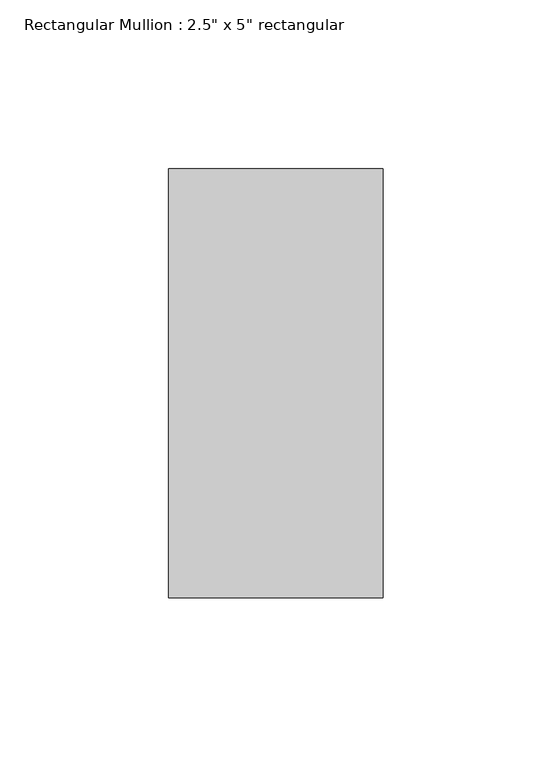
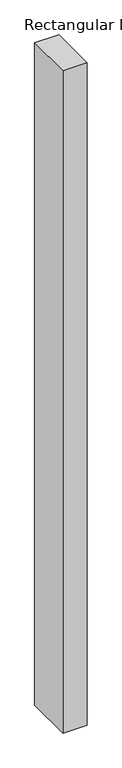
"""IFC4 building model written with IfcOpenShell, lengths in millimetres: member geometry."""

from ifc_helpers import new_model, si_unit, frame, origin, place, context, project, spatial, polyline, outline, extrude, source, transform, mapped, element, save


def member_78ce859c(model_context):
    return source(origin(), model_context, "Body", "SweptSolid", [
        extrude(outline(polyline([(31.75, 63.5), (31.75, -63.5), (-31.75, -63.5), (-31.75, 63.5), (31.75, 63.5)])), frame((0.0, 0.0, -1825.0287468), z_axis=(0.0, 0.0, 1.0), x_axis=(1.0, 0.0, 0.0)), (0.0, 0.0, 1.0), 1825.0287468),
    ])


if __name__ == "__main__":
    model = new_model("IFC4")
    model_context = context("Model", 3, world=origin())
    ifc_project = project(units=[si_unit("LENGTHUNIT", "METRE", prefix="MILLI")], contexts=[model_context])
    site = spatial("IfcSite", under=ifc_project)
    building = spatial("IfcBuilding", under=site)
    placement = place(None, origin())
    member_shape = member_78ce859c(model_context)
    element("IfcMember", 1, ObjectType="Rectangular Mullion : 2.5\" x 5\" rectangular", at=placement, inside=building, context=model_context, shape_type="MappedRepresentation", body=[
        mapped(member_shape, transform((0.0, 0.0, 0.0), x_axis=(1.0, 0.0, 0.0), y_axis=(0.0, 1.0, 0.0), z_axis=(0.0, 0.0, 1.0))),
    ])
    save(model, "model.ifc")

# Revit data of these elements
# Type "Rectangular Mullion : 2.5\" x 5\" rectangular"
#   built-in parameter 1007304 = 0.416667 (stored number, unit not read)
#   built-in parameter 1007301 = 0.104167 (stored number, unit not read)
#   built-in parameter 1007300 = 0.104167 (stored number, unit not read)
# Element 1 (IfcMember, "Rectangular Mullion : 2.5\" x 5\" rectangular")
#   Materials on its faces: "Aluminum"
# Materials
#   "Aluminum": class "Metal", colour RGB 247 247 247, transparency 0, Description = "Aluminum 6061", Cost = 0
